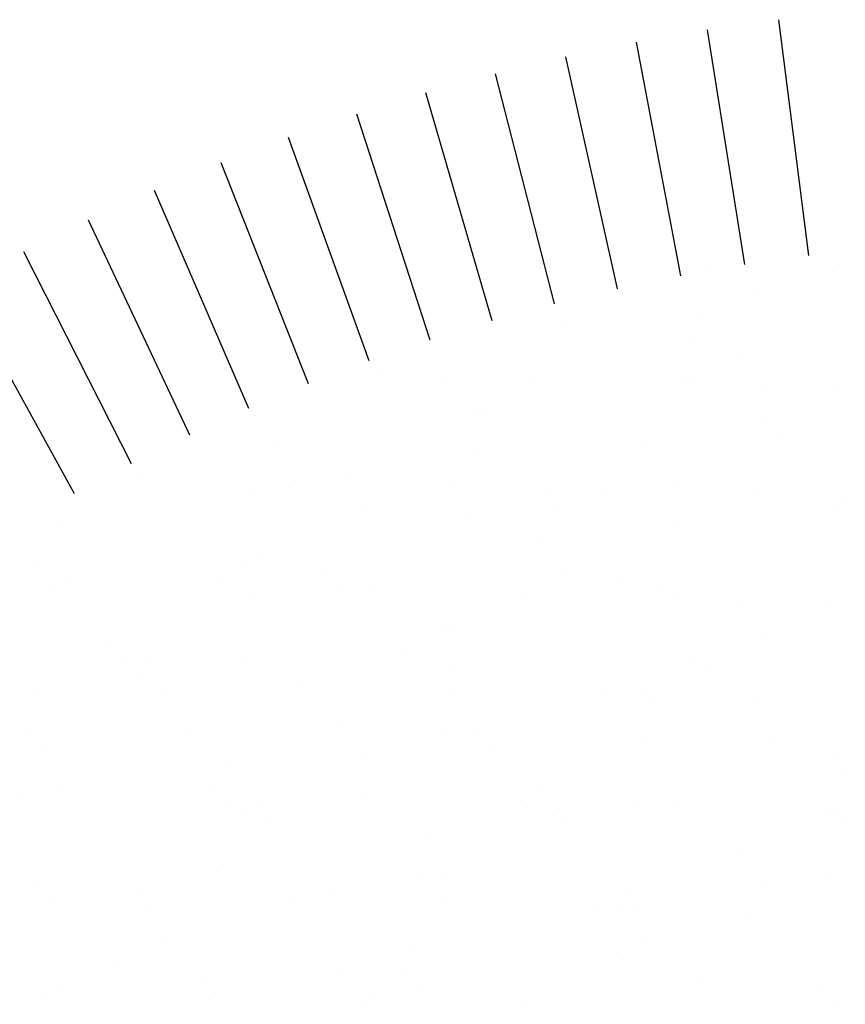
# Model space of a CAD drawing. Units: millimetres. Extents: x -857 to 54106, y -13666 to 13947.
# Tile 38 of 41: x 31622 to 32093, y 10518 to 11079. Entities that reach past the tile are written whole.
import ezdxf

# ---------------------------------------------------------------- set-up
doc = ezdxf.new("R2010")
doc.units = ezdxf.units.MM
doc.layers.add('A-FURN', color=21, linetype='Continuous', lineweight=18)
doc.layers.add('A-HT', color=15, linetype='Continuous')

# ---------------------------------------------------------------- blocks, each defined once
blk = doc.blocks.new('*X18')
at = {"color": 0}
for p, q in [((1.0527, 2.20991), (1.0527, 2.20991)), ((0.90672, 2.20023), (0.90672, 2.20023)), ((0.98603, 2.20113), (0.98603, 2.20113)), ((1.01206, 2.20456), (1.01206, 2.20456)), ((1.0214, 2.19502), (1.0214, 2.19502)), ((1.10679, 2.19851), (1.10679, 2.19851)), ((1.17711, 2.1953), (1.17711, 2.1953)), ((0.91812, 2.19219), (0.91812, 2.19219)), ((1.11601, 2.19007), (1.11601, 2.19007)), ((0.87747, 2.18684), (0.87747, 2.18684)), ((0.9137, 2.18248), (0.9137, 2.18248)), ((1.04458, 2.18415), (1.04458, 2.18415)), ((1.17249, 2.18354), (1.17249, 2.18354)), ((0.95648, 2.15463), (0.95648, 2.15463)), ((0.9657, 2.14618), (0.9657, 2.14618)), ((1.15951, 2.15021), (1.15951, 2.15021)), ((0.84924, 2.13302), (0.84924, 2.13302)), ((0.97715, 2.1324), (0.97715, 2.1324)), ((1.11219, 2.13727), (1.11219, 2.13727)), ((1.1205, 2.13188), (1.1205, 2.13188)), ((0.96479, 2.1316), (0.96479, 2.1316)), ((0.98588, 2.11817), (0.98588, 2.11817)), ((1.14159, 2.11845), (1.14159, 2.11845)), ((1.0092, 2.10633), (1.0092, 2.10633)), ((1.16672, 2.09546), (1.16672, 2.09546)), ((0.91685, 2.08614), (0.91685, 2.08614)), ((1.04773, 2.08781), (1.04773, 2.08781)), ((1.0988, 2.08652), (1.0988, 2.08652)), ((1.17564, 2.08719), (1.17564, 2.08719)), ((1.03213, 2.07775), (1.03213, 2.07775)), ((1.05816, 2.08117), (1.05816, 2.08117)), ((1.06178, 2.06981), (1.06178, 2.06981)), ((0.90608, 2.06953), (0.90608, 2.06953)), ((0.92357, 2.06345), (0.92357, 2.06345)), ((0.96422, 2.0688), (0.96422, 2.0688)), ((0.85889, 2.06244), (0.85889, 2.06244)), ((0.89754, 2.06003), (0.89754, 2.06003)), ((1.05897, 2.06072), (1.05897, 2.06072)), ((0.82963, 2.05109), (0.82963, 2.05109)), ((1.06818, 2.05228), (1.06818, 2.05228)), ((1.11534, 2.04093), (1.11534, 2.04093)), ((0.85239, 2.03668), (0.85239, 2.03668)), ((0.9803, 2.03606), (0.9803, 2.03606)), ((0.90866, 2.01684), (0.90866, 2.01684)), ((0.91788, 2.00839), (0.91788, 2.00839)), ((1.11168, 2.01242), (1.11168, 2.01242)), ((0.84947, 2.00611), (0.84947, 2.00611)), ((1.00518, 2.00639), (1.00518, 2.00639)), ((1.16088, 2.00668), (1.16088, 2.00668)), ((0.87055, 1.99268), (0.87055, 1.99268)), ((0.92, 1.9898), (0.92, 1.9898)), ((1.02626, 1.99296), (1.02626, 1.99296)), ((1.05088, 1.99147), (1.05088, 1.99147)), ((1.17879, 1.99085), (1.17879, 1.99085)), ((1.18197, 1.99324), (1.18197, 1.99324)), ((0.78496, 1.98493), (0.78496, 1.98493)), ((0.96137, 1.96853), (0.96137, 1.96853)), ((1.16145, 1.96682), (1.16145, 1.96682)), ((1.10426, 1.95778), (1.10426, 1.95778)), ((1.1449, 1.96313), (1.1449, 1.96313)), ((1.17066, 1.95837), (1.17066, 1.95837)), ((1.07823, 1.95436), (1.07823, 1.95436)), ((1.01032, 1.94542), (1.01032, 1.94542)), ((0.79075, 1.94404), (0.79075, 1.94404)), ((0.85554, 1.94034), (0.85554, 1.94034)), ((0.94646, 1.94432), (0.94646, 1.94432)), ((0.96967, 1.94006), (0.96967, 1.94006)), ((0.98345, 1.93972), (0.98345, 1.93972)), ((1.10217, 1.9446), (1.10217, 1.9446)), ((1.11849, 1.94459), (1.11849, 1.94459)), ((0.94364, 1.93664), (0.94364, 1.93664)), ((0.87573, 1.9277), (0.87573, 1.9277)), ((0.81107, 1.92465), (0.81107, 1.92465)), ((0.83508, 1.92235), (0.83508, 1.92235)), ((1.01114, 1.92293), (1.01114, 1.92293)), ((0.80905, 1.91892), (0.80905, 1.91892)), ((1.02036, 1.91449), (1.02036, 1.91449)), ((0.92315, 1.89346), (0.92315, 1.89346)), ((1.05403, 1.89513), (1.05403, 1.89513)), ((1.18194, 1.89451), (1.18194, 1.89451)), ((0.78811, 1.88859), (0.78811, 1.88859)), ((0.86083, 1.87905), (0.86083, 1.87905)), ((0.88985, 1.88091), (0.88985, 1.88091)), ((1.04556, 1.88119), (1.04556, 1.88119)), ((1.06386, 1.87463), (1.06386, 1.87463)), ((0.75523, 1.86719), (0.75523, 1.86719)), ((0.87005, 1.8706), (0.87005, 1.8706)), ((0.91093, 1.86747), (0.91093, 1.86747)), ((1.06664, 1.86776), (1.06664, 1.86776)), ((1.12164, 1.84825), (1.12164, 1.84825)), ((0.85869, 1.84399), (0.85869, 1.84399)), ((0.9866, 1.84338), (0.9866, 1.84338)), ((1.15035, 1.83439), (1.15035, 1.83439)), ((0.91355, 1.83074), (0.91355, 1.83074)), ((1.11362, 1.82902), (1.11362, 1.82902)), ((1.12433, 1.83097), (1.12433, 1.83097)), ((1.05642, 1.82203), (1.05642, 1.82203)), ((0.83113, 1.81883), (0.83113, 1.81883)), ((0.98684, 1.81912), (0.98684, 1.81912)), ((1.01577, 1.81668), (1.01577, 1.81668)), ((1.12284, 1.82058), (1.12284, 1.82058)), ((1.14255, 1.8194), (1.14255, 1.8194)), ((0.98974, 1.81325), (0.98974, 1.81325)), ((0.92183, 1.80431), (0.92183, 1.80431)), ((0.88118, 1.79896), (0.88118, 1.79896)), ((0.9263, 1.79712), (0.9263, 1.79712)), ((1.05718, 1.79878), (1.05718, 1.79878)), ((0.79126, 1.79225), (0.79126, 1.79225)), ((0.85515, 1.79553), (0.85515, 1.79553)), ((0.76324, 1.78686), (0.76324, 1.78686)), ((0.78724, 1.78659), (0.78724, 1.78659)), ((0.96332, 1.78514), (0.96332, 1.78514)), ((0.72056, 1.77781), (0.72056, 1.77781)), ((0.74659, 1.78124), (0.74659, 1.78124)), ((1.16634, 1.78072), (1.16634, 1.78072)), ((0.97253, 1.7767), (0.97253, 1.7767)), ((0.77452, 1.75542), (0.77452, 1.75542)), ((0.93023, 1.7557), (0.93023, 1.7557)), ((1.08594, 1.75598), (1.08594, 1.75598)), ((0.86184, 1.74765), (0.86184, 1.74765)), ((0.98975, 1.74704), (0.98975, 1.74704)), ((1.12479, 1.75191), (1.12479, 1.75191)), ((0.73096, 1.74598), (0.73096, 1.74598)), ((0.79561, 1.74199), (0.79561, 1.74199)), ((0.81301, 1.74126), (0.81301, 1.74126)), ((0.95132, 1.74227), (0.95132, 1.74227)), ((1.10702, 1.74255), (1.10702, 1.74255)), ((1.01603, 1.73684), (1.01603, 1.73684)), ((0.82223, 1.73281), (0.82223, 1.73281)), ((1.17043, 1.70758), (1.17043, 1.70758)), ((0.92945, 1.70077), (0.92945, 1.70077)), ((1.06033, 1.70244), (1.06033, 1.70244)), ((1.10252, 1.69864), (1.10252, 1.69864)), ((0.71581, 1.69335), (0.71581, 1.69335)), ((0.79441, 1.69591), (0.79441, 1.69591)), ((0.86573, 1.69295), (0.86573, 1.69295)), ((0.87151, 1.69363), (0.87151, 1.69363)), ((1.02722, 1.69391), (1.02722, 1.69391)), ((1.06187, 1.69329), (1.06187, 1.69329)), ((1.0658, 1.69123), (1.0658, 1.69123)), ((1.18293, 1.69419), (1.18293, 1.69419)), ((1.03584, 1.68986), (1.03584, 1.68986))]:
    blk.add_line(p, q, dxfattribs=at)
blk = doc.blocks.new('A$C6796526C')
at = {"layer": 'A-HT'}
for p, q in [((0.16025, 1.28707), (0.01143, 1.26827)), ((0.16601, 1.24664), (0.01785, 1.22317)), ((0.17303, 1.2064), (0.02568, 1.1783)), ((0.18131, 1.16641), (0.03492, 1.13369)), ((0.19084, 1.1267), (0.04555, 1.0894)), ((0.20162, 1.08731), (0.05757, 1.04546)), ((0.21363, 1.04828), (0.07097, 1.00193)), ((0.22686, 1.00964), (0.08572, 0.95883)), ((0.24129, 0.97144), (0.10182, 0.91622)), ((0.25692, 0.93371), (0.11926, 0.87414)), ((0.27373, 0.89649), (0.138, 0.83262)), ((0.29169, 0.85981), (0.15804, 0.79171)), ((0.3108, 0.82372), (0.17936, 0.75146))]:
    blk.add_line(p, q, dxfattribs=at)
at = {"layer": 'A-HT', "extrusion": (0, 0, -1), "zscale": -1, "rotation": 180}
blk.add_blockref('*X18', (0.55, 3), dxfattribs=at)

msp = doc.modelspace()

# ---------------------------------------------------------------- block references
at = {"layer": 'A-FURN', "xscale": 903.6084929786902, "yscale": 903.6084929786902, "zscale": 903.6084929786902, "rotation": 269.9999999999988}
msp.add_blockref('A$C6796526C', (30909.253, 11089.463), dxfattribs=at)

doc.saveas('drawing.dxf')
